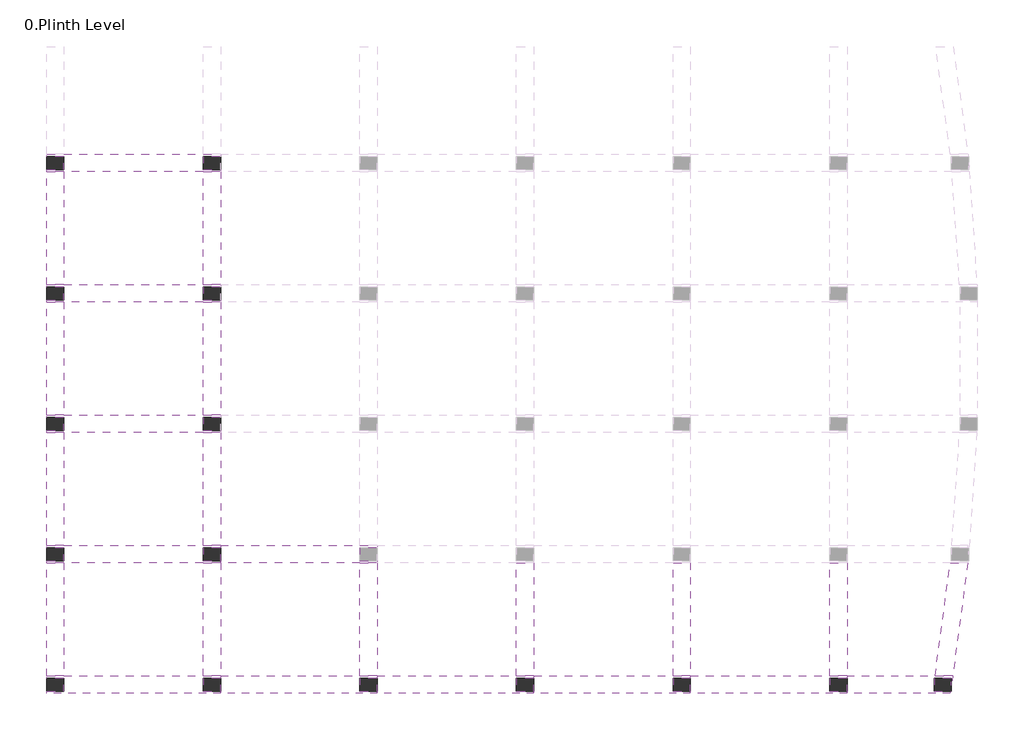
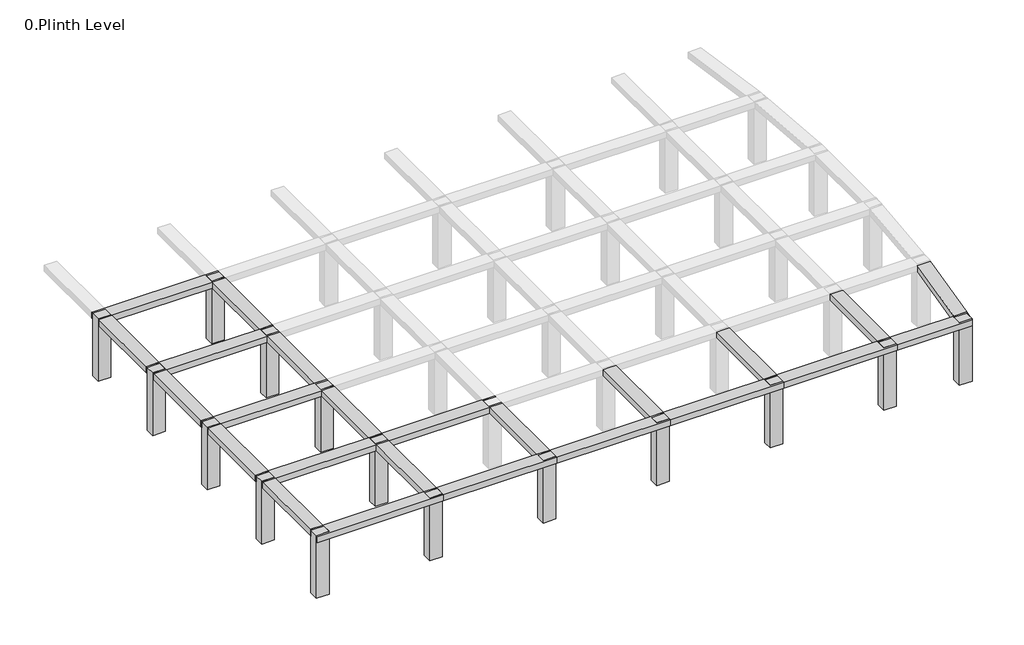
# One storey, part 1 of 3: 24 beams, 15 columns.
"""IFC4 building model written with IfcOpenShell, lengths in millimetres."""

from ifc_helpers import new_model, si_unit, frame, origin, origin_with_axes, place, context, project, spatial, polyline, outline, extrude, faceted_brep, element, save

model = new_model("IFC4")

# Units and contexts
model_context = context("Model", 3, world=origin())
ifc_project = project(units=[si_unit("LENGTHUNIT", "METRE", prefix="MILLI")], contexts=[model_context])

# Site, building, storey
site = spatial("IfcSite", under=ifc_project)
building = spatial("IfcBuilding", under=site)
storey = spatial("IfcBuildingStorey", under=building, Name="0.Plinth Level", Elevation=0.0)

# Beams
placement = place(None, origin())
element("IfcBeam", 1, ObjectType="Concrete-Rectangular Beam : 2' x2'", at=placement, inside=storey, context=model_context, shape_type="Brep", body=[
    faceted_brep([(-16619.274232, -2891.2168778, 3200.4), (-17228.874232, -2891.2168778, 3200.4), (-22105.674232, -2891.2168778, 3200.4), (-22715.274232, -2891.2168778, 3200.4), (-22715.274232, -2967.4168778, 3200.4), (-22105.674232, -2967.4168778, 3200.4), (-22105.674232, -3424.6168778, 3200.4), (-22715.274232, -3424.6168778, 3200.4), (-22715.274232, -3500.8168778, 3200.4), (-16619.274232, -3500.8168778, 3200.4), (-16619.274232, -3424.6168778, 3200.4), (-17228.874232, -3424.6168778, 3200.4), (-17228.874232, -2967.4168778, 3200.4), (-16619.274232, -2967.4168778, 3200.4), (-22715.274232, -3500.8168778, 2895.6), (-16619.274232, -3500.8168778, 2895.6), (-22715.274232, -3424.6168778, 2895.6), (-22105.674232, -3424.6168778, 2895.6), (-22105.674232, -2967.4168778, 2895.6), (-22715.274232, -2967.4168778, 2895.6), (-22715.274232, -2891.2168778, 2895.6), (-22105.674232, -2891.2168778, 2895.6), (-17228.874232, -2891.2168778, 2895.6), (-16619.274232, -2891.2168778, 2895.6), (-16619.274232, -2967.4168778, 2895.6), (-17228.874232, -2967.4168778, 2895.6), (-17228.874232, -3424.6168778, 2895.6), (-16619.274232, -3424.6168778, 2895.6)], [[[0, 1, 2, 3, 4, 5, 6, 7, 8, 9, 10, 11, 12, 13]], [[8, 14, 15, 9]], [[15, 14, 16, 17, 18, 19, 20, 21, 22, 23, 24, 25, 26, 27]], [[20, 3, 2, 1, 0, 23, 22, 21]], [[14, 8, 7, 16]], [[9, 15, 27, 10]], [[17, 6, 5, 18]], [[6, 17, 16, 7]], [[18, 5, 4, 19]], [[3, 20, 19, 4]], [[26, 11, 10, 27]], [[11, 26, 25, 12]], [[12, 25, 24, 13]], [[23, 0, 13, 24]]]),
])
element("IfcBeam", 2, ObjectType="Concrete-Rectangular Beam : 2' x2'", at=placement, inside=storey, context=model_context, shape_type="Brep", body=[
    faceted_brep([(-16619.274232, -2891.2168778, 3200.4), (-16619.274232, -2967.4168778, 3200.4), (-16619.274232, -3424.6168778, 3200.4), (-16619.274232, -3500.8168778, 3200.4), (-11132.874232, -3500.8168778, 3200.4), (-11132.874232, -3424.6168778, 3200.4), (-11742.474232, -3424.6168778, 3200.4), (-11742.474232, -2967.4168778, 3200.4), (-11132.874232, -2967.4168778, 3200.4), (-11132.874232, -2891.2168778, 3200.4), (-11742.474232, -2891.2168778, 3200.4), (-11132.874232, -3500.8168778, 2895.6), (-16619.274232, -3500.8168778, 2895.6), (-16619.274232, -3424.6168778, 2895.6), (-16619.274232, -2967.4168778, 2895.6), (-16619.274232, -2891.2168778, 2895.6), (-11742.474232, -2891.2168778, 2895.6), (-11132.874232, -2891.2168778, 2895.6), (-11132.874232, -2967.4168778, 2895.6), (-11742.474232, -2967.4168778, 2895.6), (-11742.474232, -3424.6168778, 2895.6), (-11132.874232, -3424.6168778, 2895.6)], [[[0, 1, 2, 3, 4, 5, 6, 7, 8, 9, 10]], [[11, 4, 3, 12]], [[12, 13, 14, 15, 16, 17, 18, 19, 20, 21, 11]], [[15, 0, 10, 9, 17, 16]], [[3, 2, 1, 0, 15, 14, 13, 12]], [[4, 11, 21, 5]], [[20, 6, 5, 21]], [[6, 20, 19, 7]], [[7, 19, 18, 8]], [[17, 9, 8, 18]]]),
])
element("IfcBeam", 3, ObjectType="Concrete-Rectangular Beam : 2' x2'", at=placement, inside=storey, context=model_context, shape_type="Brep", body=[
    faceted_brep([(-5646.474232, -2891.2168778, 3200.4), (-6256.074232, -2891.2168778, 3200.4), (-11132.874232, -2891.2168778, 3200.4), (-11132.874232, -2967.4168778, 3200.4), (-11132.874232, -3424.6168778, 3200.4), (-11132.874232, -3500.8168778, 3200.4), (-5646.474232, -3500.8168778, 3200.4), (-5646.474232, -3424.6168778, 3200.4), (-6256.074232, -3424.6168778, 3200.4), (-6256.074232, -2967.4168778, 3200.4), (-5646.474232, -2967.4168778, 3200.4), (-5646.474232, -3500.8168778, 2895.6), (-11132.874232, -3500.8168778, 2895.6), (-11132.874232, -3424.6168778, 2895.6), (-11132.874232, -2967.4168778, 2895.6), (-11132.874232, -2891.2168778, 2895.6), (-6256.074232, -2891.2168778, 2895.6), (-5646.474232, -2891.2168778, 2895.6), (-5646.474232, -2967.4168778, 2895.6), (-6256.074232, -2967.4168778, 2895.6), (-6256.074232, -3424.6168778, 2895.6), (-5646.474232, -3424.6168778, 2895.6)], [[[0, 1, 2, 3, 4, 5, 6, 7, 8, 9, 10]], [[11, 6, 5, 12]], [[11, 12, 13, 14, 15, 16, 17, 18, 19, 20, 21]], [[0, 17, 16, 15, 2, 1]], [[6, 11, 21, 7]], [[5, 4, 3, 2, 15, 14, 13, 12]], [[20, 8, 7, 21]], [[8, 20, 19, 9]], [[9, 19, 18, 10]], [[17, 0, 10, 18]]]),
])
element("IfcBeam", 4, ObjectType="Concrete-Rectangular Beam : 2' x2'", at=placement, inside=storey, context=model_context, shape_type="Brep", body=[
    faceted_brep([(-5646.474232, -2891.2168778, 3200.4), (-5646.474232, -2967.4168778, 3200.4), (-5646.474232, -3424.6168778, 3200.4), (-5646.474232, -3500.8168778, 3200.4), (-160.074232, -3500.8168778, 3200.4), (-160.074232, -3424.6168778, 3200.4), (-769.674232, -3424.6168778, 3200.4), (-769.674232, -2967.4168778, 3200.4), (-160.074232, -2967.4168778, 3200.4), (-160.074232, -2891.2168778, 3200.4), (-769.674232, -2891.2168778, 3200.4), (-160.074232, -3500.8168778, 2895.6), (-5646.474232, -3500.8168778, 2895.6), (-5646.474232, -3424.6168778, 2895.6), (-5646.474232, -2967.4168778, 2895.6), (-5646.474232, -2891.2168778, 2895.6), (-769.674232, -2891.2168778, 2895.6), (-160.074232, -2891.2168778, 2895.6), (-160.074232, -2967.4168778, 2895.6), (-769.674232, -2967.4168778, 2895.6), (-769.674232, -3424.6168778, 2895.6), (-160.074232, -3424.6168778, 2895.6)], [[[0, 1, 2, 3, 4, 5, 6, 7, 8, 9, 10]], [[11, 4, 3, 12]], [[12, 13, 14, 15, 16, 17, 18, 19, 20, 21, 11]], [[15, 0, 10, 9, 17, 16]], [[3, 2, 1, 0, 15, 14, 13, 12]], [[4, 11, 21, 5]], [[20, 6, 5, 21]], [[6, 20, 19, 7]], [[7, 19, 18, 8]], [[17, 9, 8, 18]]]),
])
element("IfcBeam", 5, ObjectType="Concrete-Rectangular Beam : 2' x2'", at=placement, inside=storey, context=model_context, shape_type="Brep", body=[
    faceted_brep([(-160.074232, -2891.2168778, 3200.4), (-160.074232, -2967.4168778, 3200.4), (-160.074232, -3424.6168778, 3200.4), (-160.074232, -3500.8168778, 3200.4), (5326.325768, -3500.8168778, 3200.4), (5326.325768, -3424.6168778, 3200.4), (4716.725768, -3424.6168778, 3200.4), (4716.725768, -2967.4168778, 3200.4), (5326.325768, -2967.4168778, 3200.4), (5326.325768, -2891.2168778, 3200.4), (4716.725768, -2891.2168778, 3200.4), (5326.325768, -3500.8168778, 2895.6), (-160.074232, -3500.8168778, 2895.6), (-160.074232, -3424.6168778, 2895.6), (-160.074232, -2967.4168778, 2895.6), (-160.074232, -2891.2168778, 2895.6), (4716.725768, -2891.2168778, 2895.6), (5326.325768, -2891.2168778, 2895.6), (5326.325768, -2967.4168778, 2895.6), (4716.725768, -2967.4168778, 2895.6), (4716.725768, -3424.6168778, 2895.6), (5326.325768, -3424.6168778, 2895.6)], [[[0, 1, 2, 3, 4, 5, 6, 7, 8, 9, 10]], [[11, 4, 3, 12]], [[12, 13, 14, 15, 16, 17, 18, 19, 20, 21, 11]], [[15, 0, 10, 9, 17, 16]], [[3, 2, 1, 0, 15, 14, 13, 12]], [[4, 11, 21, 5]], [[20, 6, 5, 21]], [[6, 20, 19, 7]], [[7, 19, 18, 8]], [[17, 9, 8, 18]]]),
])
element("IfcBeam", 6, ObjectType="Concrete-Rectangular Beam : 2' x2'", at=placement, inside=storey, context=model_context, shape_type="Brep", body=[
    faceted_brep([(9027.2344863, -2891.2168778, 3200.4), (8412.2463849, -2891.2168778, 3200.4), (5326.325768, -2891.2168778, 3200.4), (5326.325768, -2967.4168778, 3200.4), (5326.325768, -3424.6168778, 3200.4), (5326.325768, -3500.8168778, 3200.4), (8946.005151, -3500.8168778, 3200.4), (8956.158818, -3424.6168778, 3200.4), (8374.325768, -3424.6168778, 3200.4), (8374.325768, -2967.4168778, 3200.4), (8983.925768, -2967.4168778, 3200.4), (8983.925768, -3216.2348608, 3200.4), (8946.005151, -3500.8168778, 2895.6), (5326.325768, -3500.8168778, 2895.6), (5326.325768, -3424.6168778, 2895.6), (5326.325768, -2967.4168778, 2895.6), (5326.325768, -2891.2168778, 2895.6), (8412.2463849, -2891.2168778, 2895.6), (9027.2344863, -2891.2168778, 2895.6), (8983.925768, -3216.2348608, 2895.6), (8983.925768, -2967.4168778, 2895.6), (8374.325768, -2967.4168778, 2895.6), (8374.325768, -3424.6168778, 2895.6), (8956.158818, -3424.6168778, 2895.6)], [[[0, 1, 2, 3, 4, 5, 6, 7, 8, 9, 10, 11]], [[12, 6, 5, 13]], [[12, 13, 14, 15, 16, 17, 18, 19, 20, 21, 22, 23]], [[0, 18, 17, 16, 2, 1]], [[6, 12, 23, 7]], [[5, 4, 3, 2, 16, 15, 14, 13]], [[10, 20, 19, 11]], [[22, 8, 7, 23]], [[8, 22, 21, 9]], [[9, 21, 20, 10]], [[18, 0, 11, 19]]]),
])
element("IfcBeam", 7, ObjectType="Concrete-Rectangular Beam : 2' x2'", at=placement, inside=storey, context=model_context, shape_type="Brep", body=[
    faceted_brep([(-16619.274232, 1680.7831222, 3200.4), (-17228.874232, 1680.7831222, 3200.4), (-22105.674232, 1680.7831222, 3200.4), (-22715.274232, 1680.7831222, 3200.4), (-22715.274232, 1604.5831222, 3200.4), (-22105.674232, 1604.5831222, 3200.4), (-22105.674232, 1147.3831222, 3200.4), (-22715.274232, 1147.3831222, 3200.4), (-22715.274232, 1071.1831222, 3200.4), (-22105.674232, 1071.1831222, 3200.4), (-17228.874232, 1071.1831222, 3200.4), (-16619.274232, 1071.1831222, 3200.4), (-16619.274232, 1147.3831222, 3200.4), (-17228.874232, 1147.3831222, 3200.4), (-17228.874232, 1604.5831222, 3200.4), (-16619.274232, 1604.5831222, 3200.4), (-22715.274232, 1071.1831222, 2895.6), (-22105.674232, 1071.1831222, 2895.6), (-17228.874232, 1071.1831222, 2895.6), (-16619.274232, 1071.1831222, 2895.6), (-22715.274232, 1147.3831222, 2895.6), (-22105.674232, 1147.3831222, 2895.6), (-22105.674232, 1604.5831222, 2895.6), (-22715.274232, 1604.5831222, 2895.6), (-22715.274232, 1680.7831222, 2895.6), (-22105.674232, 1680.7831222, 2895.6), (-17228.874232, 1680.7831222, 2895.6), (-16619.274232, 1680.7831222, 2895.6), (-16619.274232, 1604.5831222, 2895.6), (-17228.874232, 1604.5831222, 2895.6), (-17228.874232, 1147.3831222, 2895.6), (-16619.274232, 1147.3831222, 2895.6)], [[[0, 1, 2, 3, 4, 5, 6, 7, 8, 9, 10, 11, 12, 13, 14, 15]], [[8, 16, 17, 18, 19, 11, 10, 9]], [[19, 18, 17, 16, 20, 21, 22, 23, 24, 25, 26, 27, 28, 29, 30, 31]], [[24, 3, 2, 1, 0, 27, 26, 25]], [[16, 8, 7, 20]], [[11, 19, 31, 12]], [[21, 6, 5, 22]], [[6, 21, 20, 7]], [[22, 5, 4, 23]], [[3, 24, 23, 4]], [[30, 13, 12, 31]], [[13, 30, 29, 14]], [[14, 29, 28, 15]], [[27, 0, 15, 28]]]),
])
element("IfcBeam", 8, ObjectType="Concrete-Rectangular Beam : 2' x2'", at=placement, inside=storey, context=model_context, shape_type="Brep", body=[
    faceted_brep([(-16619.274232, 1680.7831222, 3200.4), (-16619.274232, 1604.5831222, 3200.4), (-16619.274232, 1147.3831222, 3200.4), (-16619.274232, 1071.1831222, 3200.4), (-11742.474232, 1071.1831222, 3200.4), (-11132.874232, 1071.1831222, 3200.4), (-11132.874232, 1147.3831222, 3200.4), (-11742.474232, 1147.3831222, 3200.4), (-11742.474232, 1604.5831222, 3200.4), (-11132.874232, 1604.5831222, 3200.4), (-11132.874232, 1680.7831222, 3200.4), (-11742.474232, 1680.7831222, 3200.4), (-16619.274232, 1071.1831222, 2895.6), (-11742.474232, 1071.1831222, 2895.6), (-11132.874232, 1071.1831222, 2895.6), (-16619.274232, 1147.3831222, 2895.6), (-16619.274232, 1604.5831222, 2895.6), (-16619.274232, 1680.7831222, 2895.6), (-11742.474232, 1680.7831222, 2895.6), (-11132.874232, 1680.7831222, 2895.6), (-11132.874232, 1604.5831222, 2895.6), (-11742.474232, 1604.5831222, 2895.6), (-11742.474232, 1147.3831222, 2895.6), (-11132.874232, 1147.3831222, 2895.6)], [[[0, 1, 2, 3, 4, 5, 6, 7, 8, 9, 10, 11]], [[3, 12, 13, 14, 5, 4]], [[12, 15, 16, 17, 18, 19, 20, 21, 22, 23, 14, 13]], [[10, 19, 18, 17, 0, 11]], [[3, 2, 1, 0, 17, 16, 15, 12]], [[5, 14, 23, 6]], [[22, 7, 6, 23]], [[7, 22, 21, 8]], [[8, 21, 20, 9]], [[19, 10, 9, 20]]]),
])
element("IfcBeam", 9, ObjectType="Concrete-Rectangular Beam : 2' x2'", at=placement, inside=storey, context=model_context, shape_type="Brep", body=[
    faceted_brep([(-16619.274232, 6252.7831222, 3200.4), (-17228.874232, 6252.7831222, 3200.4), (-22105.674232, 6252.7831222, 3200.4), (-22715.274232, 6252.7831222, 3200.4), (-22715.274232, 6176.5831222, 3200.4), (-22105.674232, 6176.5831222, 3200.4), (-22105.674232, 5719.3831222, 3200.4), (-22715.274232, 5719.3831222, 3200.4), (-22715.274232, 5643.1831222, 3200.4), (-22105.674232, 5643.1831222, 3200.4), (-17228.874232, 5643.1831222, 3200.4), (-16619.274232, 5643.1831222, 3200.4), (-16619.274232, 5719.3831222, 3200.4), (-17228.874232, 5719.3831222, 3200.4), (-17228.874232, 6176.5831222, 3200.4), (-16619.274232, 6176.5831222, 3200.4), (-22715.274232, 5643.1831222, 2895.6), (-22105.674232, 5643.1831222, 2895.6), (-17228.874232, 5643.1831222, 2895.6), (-16619.274232, 5643.1831222, 2895.6), (-22715.274232, 5719.3831222, 2895.6), (-22105.674232, 5719.3831222, 2895.6), (-22105.674232, 6176.5831222, 2895.6), (-22715.274232, 6176.5831222, 2895.6), (-22715.274232, 6252.7831222, 2895.6), (-22105.674232, 6252.7831222, 2895.6), (-17228.874232, 6252.7831222, 2895.6), (-16619.274232, 6252.7831222, 2895.6), (-16619.274232, 6176.5831222, 2895.6), (-17228.874232, 6176.5831222, 2895.6), (-17228.874232, 5719.3831222, 2895.6), (-16619.274232, 5719.3831222, 2895.6)], [[[0, 1, 2, 3, 4, 5, 6, 7, 8, 9, 10, 11, 12, 13, 14, 15]], [[8, 16, 17, 18, 19, 11, 10, 9]], [[19, 18, 17, 16, 20, 21, 22, 23, 24, 25, 26, 27, 28, 29, 30, 31]], [[24, 3, 2, 1, 0, 27, 26, 25]], [[16, 8, 7, 20]], [[11, 19, 31, 12]], [[21, 6, 5, 22]], [[6, 21, 20, 7]], [[22, 5, 4, 23]], [[3, 24, 23, 4]], [[30, 13, 12, 31]], [[13, 30, 29, 14]], [[14, 29, 28, 15]], [[27, 0, 15, 28]]]),
])
element("IfcBeam", 10, ObjectType="Concrete-Rectangular Beam : 2' x2'", at=placement, inside=storey, context=model_context, shape_type="Brep", body=[
    faceted_brep([(-16619.274232, 10824.7831222, 3200.4), (-17228.874232, 10824.7831222, 3200.4), (-22105.674232, 10824.7831222, 3200.4), (-22715.274232, 10824.7831222, 3200.4), (-22715.274232, 10748.5831222, 3200.4), (-22105.674232, 10748.5831222, 3200.4), (-22105.674232, 10291.3831222, 3200.4), (-22715.274232, 10291.3831222, 3200.4), (-22715.274232, 10215.1831222, 3200.4), (-22105.674232, 10215.1831222, 3200.4), (-17228.874232, 10215.1831222, 3200.4), (-16619.274232, 10215.1831222, 3200.4), (-16619.274232, 10291.3831222, 3200.4), (-17228.874232, 10291.3831222, 3200.4), (-17228.874232, 10748.5831222, 3200.4), (-16619.274232, 10748.5831222, 3200.4), (-22715.274232, 10215.1831222, 2895.6), (-22105.674232, 10215.1831222, 2895.6), (-17228.874232, 10215.1831222, 2895.6), (-16619.274232, 10215.1831222, 2895.6), (-22715.274232, 10291.3831222, 2895.6), (-22105.674232, 10291.3831222, 2895.6), (-22105.674232, 10748.5831222, 2895.6), (-22715.274232, 10748.5831222, 2895.6), (-22715.274232, 10824.7831222, 2895.6), (-22105.674232, 10824.7831222, 2895.6), (-17228.874232, 10824.7831222, 2895.6), (-16619.274232, 10824.7831222, 2895.6), (-16619.274232, 10748.5831222, 2895.6), (-17228.874232, 10748.5831222, 2895.6), (-17228.874232, 10291.3831222, 2895.6), (-16619.274232, 10291.3831222, 2895.6)], [[[0, 1, 2, 3, 4, 5, 6, 7, 8, 9, 10, 11, 12, 13, 14, 15]], [[8, 16, 17, 18, 19, 11, 10, 9]], [[19, 18, 17, 16, 20, 21, 22, 23, 24, 25, 26, 27, 28, 29, 30, 31]], [[24, 3, 2, 1, 0, 27, 26, 25]], [[16, 8, 7, 20]], [[11, 19, 31, 12]], [[21, 6, 5, 22]], [[6, 21, 20, 7]], [[22, 5, 4, 23]], [[3, 24, 23, 4]], [[30, 13, 12, 31]], [[13, 30, 29, 14]], [[14, 29, 28, 15]], [[27, 0, 15, 28]]]),
])
element("IfcBeam", 11, ObjectType="Concrete-Rectangular Beam : 2' x2'", at=placement, inside=storey, context=model_context, shape_type="Brep", body=[
    faceted_brep([(-16619.274232, 15396.7831222, 3200.4), (-17228.874232, 15396.7831222, 3200.4), (-22105.674232, 15396.7831222, 3200.4), (-22715.274232, 15396.7831222, 3200.4), (-22715.274232, 15320.5831222, 3200.4), (-22105.674232, 15320.5831222, 3200.4), (-22105.674232, 14863.3831222, 3200.4), (-22715.274232, 14863.3831222, 3200.4), (-22715.274232, 14787.1831222, 3200.4), (-22105.674232, 14787.1831222, 3200.4), (-17228.874232, 14787.1831222, 3200.4), (-16619.274232, 14787.1831222, 3200.4), (-16619.274232, 14863.3831222, 3200.4), (-17228.874232, 14863.3831222, 3200.4), (-17228.874232, 15320.5831222, 3200.4), (-16619.274232, 15320.5831222, 3200.4), (-22715.274232, 14787.1831222, 2895.6), (-22105.674232, 14787.1831222, 2895.6), (-17228.874232, 14787.1831222, 2895.6), (-16619.274232, 14787.1831222, 2895.6), (-22715.274232, 14863.3831222, 2895.6), (-22105.674232, 14863.3831222, 2895.6), (-22105.674232, 15320.5831222, 2895.6), (-22715.274232, 15320.5831222, 2895.6), (-22715.274232, 15396.7831222, 2895.6), (-22105.674232, 15396.7831222, 2895.6), (-17228.874232, 15396.7831222, 2895.6), (-16619.274232, 15396.7831222, 2895.6), (-16619.274232, 15320.5831222, 2895.6), (-17228.874232, 15320.5831222, 2895.6), (-17228.874232, 14863.3831222, 2895.6), (-16619.274232, 14863.3831222, 2895.6)], [[[0, 1, 2, 3, 4, 5, 6, 7, 8, 9, 10, 11, 12, 13, 14, 15]], [[8, 16, 17, 18, 19, 11, 10, 9]], [[19, 18, 17, 16, 20, 21, 22, 23, 24, 25, 26, 27, 28, 29, 30, 31]], [[24, 3, 2, 1, 0, 27, 26, 25]], [[16, 8, 7, 20]], [[11, 19, 31, 12]], [[21, 6, 5, 22]], [[6, 21, 20, 7]], [[22, 5, 4, 23]], [[3, 24, 23, 4]], [[30, 13, 12, 31]], [[13, 30, 29, 14]], [[14, 29, 28, 15]], [[27, 0, 15, 28]]]),
])
element("IfcBeam", 12, ObjectType="Concrete-Rectangular Beam : 2' x2'", at=placement, inside=storey, context=model_context, shape_type="SweptSolid", body=[
    extrude(outline(polyline([(-22105.674232, -2891.2168778), (-22715.274232, -2891.2168778), (-22715.274232, 1071.1831222), (-22105.674232, 1071.1831222), (-22105.674232, -2891.2168778)])), frame((0.0, 0.0, 2895.6), z_axis=(0.0, 0.0, 1.0), x_axis=(1.0, 0.0, 0.0)), (0.0, 0.0, 1.0), 304.8),
])
element("IfcBeam", 13, ObjectType="Concrete-Rectangular Beam : 2' x2'", at=placement, inside=storey, context=model_context, shape_type="SweptSolid", body=[
    extrude(outline(polyline([(-22105.674232, 1680.7831222), (-22715.274232, 1680.7831222), (-22715.274232, 5643.1831222), (-22105.674232, 5643.1831222), (-22105.674232, 1680.7831222)])), frame((0.0, 0.0, 2895.6), z_axis=(0.0, 0.0, 1.0), x_axis=(1.0, 0.0, 0.0)), (0.0, 0.0, 1.0), 304.8),
])
element("IfcBeam", 14, ObjectType="Concrete-Rectangular Beam : 2' x2'", at=placement, inside=storey, context=model_context, shape_type="SweptSolid", body=[
    extrude(outline(polyline([(-22105.674232, 6252.7831222), (-22715.274232, 6252.7831222), (-22715.274232, 10215.1831222), (-22105.674232, 10215.1831222), (-22105.674232, 6252.7831222)])), frame((0.0, 0.0, 2895.6), z_axis=(0.0, 0.0, 1.0), x_axis=(1.0, 0.0, 0.0)), (0.0, 0.0, 1.0), 304.8),
])
element("IfcBeam", 15, ObjectType="Concrete-Rectangular Beam : 2' x2'", at=placement, inside=storey, context=model_context, shape_type="SweptSolid", body=[
    extrude(outline(polyline([(-22105.674232, 10824.7831222), (-22715.274232, 10824.7831222), (-22715.274232, 14787.1831222), (-22105.674232, 14787.1831222), (-22105.674232, 10824.7831222)])), frame((0.0, 0.0, 2895.6), z_axis=(0.0, 0.0, 1.0), x_axis=(1.0, 0.0, 0.0)), (0.0, 0.0, 1.0), 304.8),
])
element("IfcBeam", 16, ObjectType="Concrete-Rectangular Beam : 2' x2'", at=placement, inside=storey, context=model_context, shape_type="SweptSolid", body=[
    extrude(outline(polyline([(-17228.874232, 1071.1831222), (-16619.274232, 1071.1831222), (-16619.274232, -2891.2168778), (-17228.874232, -2891.2168778), (-17228.874232, 1071.1831222)])), frame((0.0, 0.0, 2895.6), z_axis=(0.0, 0.0, 1.0), x_axis=(1.0, 0.0, 0.0)), (0.0, 0.0, 1.0), 304.8),
])
element("IfcBeam", 17, ObjectType="Concrete-Rectangular Beam : 2' x2'", at=placement, inside=storey, context=model_context, shape_type="SweptSolid", body=[
    extrude(outline(polyline([(-16619.274232, 1680.7831222), (-17228.874232, 1680.7831222), (-17228.874232, 5643.1831222), (-16619.274232, 5643.1831222), (-16619.274232, 1680.7831222)])), frame((0.0, 0.0, 2895.6), z_axis=(0.0, 0.0, 1.0), x_axis=(1.0, 0.0, 0.0)), (0.0, 0.0, 1.0), 304.8),
])
element("IfcBeam", 18, ObjectType="Concrete-Rectangular Beam : 2' x2'", at=placement, inside=storey, context=model_context, shape_type="SweptSolid", body=[
    extrude(outline(polyline([(-16619.274232, 6252.7831222), (-17228.874232, 6252.7831222), (-17228.874232, 10215.1831222), (-16619.274232, 10215.1831222), (-16619.274232, 6252.7831222)])), frame((0.0, 0.0, 2895.6), z_axis=(0.0, 0.0, 1.0), x_axis=(1.0, 0.0, 0.0)), (0.0, 0.0, 1.0), 304.8),
])
element("IfcBeam", 19, ObjectType="Concrete-Rectangular Beam : 2' x2'", at=placement, inside=storey, context=model_context, shape_type="SweptSolid", body=[
    extrude(outline(polyline([(-16619.274232, 10824.7831222), (-17228.874232, 10824.7831222), (-17228.874232, 14787.1831222), (-16619.274232, 14787.1831222), (-16619.274232, 10824.7831222)])), frame((0.0, 0.0, 2895.6), z_axis=(0.0, 0.0, 1.0), x_axis=(1.0, 0.0, 0.0)), (0.0, 0.0, 1.0), 304.8),
])
element("IfcBeam", 20, ObjectType="Concrete-Rectangular Beam : 2' x2'", at=placement, inside=storey, context=model_context, shape_type="SweptSolid", body=[
    extrude(outline(polyline([(-11742.474232, 1071.1831222), (-11132.874232, 1071.1831222), (-11132.874232, -2891.2168778), (-11742.474232, -2891.2168778), (-11742.474232, 1071.1831222)])), frame((0.0, 0.0, 2895.6), z_axis=(0.0, 0.0, 1.0), x_axis=(1.0, 0.0, 0.0)), (0.0, 0.0, 1.0), 304.8),
])
element("IfcBeam", 21, ObjectType="Concrete-Rectangular Beam : 2' x2'", at=placement, inside=storey, context=model_context, shape_type="SweptSolid", body=[
    extrude(outline(polyline([(-6256.074232, 1071.1831222), (-5646.474232, 1071.1831222), (-5646.474232, -2891.2168778), (-6256.074232, -2891.2168778), (-6256.074232, 1071.1831222)])), frame((0.0, 0.0, 2895.6), z_axis=(0.0, 0.0, 1.0), x_axis=(1.0, 0.0, 0.0)), (0.0, 0.0, 1.0), 304.8),
])
element("IfcBeam", 22, ObjectType="Concrete-Rectangular Beam : 2' x2'", at=placement, inside=storey, context=model_context, shape_type="SweptSolid", body=[
    extrude(outline(polyline([(-769.674232, 1071.1831222), (-160.074232, 1071.1831222), (-160.074232, -2891.2168778), (-769.674232, -2891.2168778), (-769.674232, 1071.1831222)])), frame((0.0, 0.0, 2895.6), z_axis=(0.0, 0.0, 1.0), x_axis=(1.0, 0.0, 0.0)), (0.0, 0.0, 1.0), 304.8),
])
element("IfcBeam", 23, ObjectType="Concrete-Rectangular Beam : 2' x2'", at=placement, inside=storey, context=model_context, shape_type="SweptSolid", body=[
    extrude(outline(polyline([(4716.725768, 1071.1831222), (5326.325768, 1071.1831222), (5326.325768, -2891.2168778), (4716.725768, -2891.2168778), (4716.725768, 1071.1831222)])), frame((0.0, 0.0, 2895.6), z_axis=(0.0, 0.0, 1.0), x_axis=(1.0, 0.0, 0.0)), (0.0, 0.0, 1.0), 304.8),
])
element("IfcBeam", 24, ObjectType="Concrete-Rectangular Beam : 2' x2'", at=placement, inside=storey, context=model_context, shape_type="SweptSolid", body=[
    extrude(outline(polyline([(8940.2370643, 1071.1831222), (9555.2251658, 1071.1831222), (9027.2344863, -2891.2168778), (8412.2463849, -2891.2168778), (8940.2370643, 1071.1831222)])), frame((0.0, 0.0, 2895.6), z_axis=(0.0, 0.0, 1.0), x_axis=(1.0, 0.0, 0.0)), (0.0, 0.0, 1.0), 304.8),
])

# Columns
element("IfcColumn", 25, ObjectType="Concrete-Rectangular-Column : 12 x 18", at=placement, inside=storey, context=model_context, shape_type="SweptSolid", body=[
    extrude(outline(polyline([(-22105.674232, -2967.4168778), (-22105.674232, -3424.6168778), (-22715.274232, -3424.6168778), (-22715.274232, -2967.4168778), (-22105.674232, -2967.4168778)])), origin_with_axes(), (0.0, 0.0, 1.0), 3200.4),
])
element("IfcColumn", 26, ObjectType="Concrete-Rectangular-Column : 12 x 18", at=placement, inside=storey, context=model_context, shape_type="SweptSolid", body=[
    extrude(outline(polyline([(-16619.274232, -2967.4168778), (-16619.274232, -3424.6168778), (-17228.874232, -3424.6168778), (-17228.874232, -2967.4168778), (-16619.274232, -2967.4168778)])), origin_with_axes(), (0.0, 0.0, 1.0), 3200.4),
])
element("IfcColumn", 27, ObjectType="Concrete-Rectangular-Column : 12 x 18", at=placement, inside=storey, context=model_context, shape_type="SweptSolid", body=[
    extrude(outline(polyline([(-11132.874232, -2967.4168778), (-11132.874232, -3424.6168778), (-11742.474232, -3424.6168778), (-11742.474232, -2967.4168778), (-11132.874232, -2967.4168778)])), origin_with_axes(), (0.0, 0.0, 1.0), 3200.4),
])
element("IfcColumn", 28, ObjectType="Concrete-Rectangular-Column : 12 x 18", at=placement, inside=storey, context=model_context, shape_type="SweptSolid", body=[
    extrude(outline(polyline([(-5646.474232, -2967.4168778), (-5646.474232, -3424.6168778), (-6256.074232, -3424.6168778), (-6256.074232, -2967.4168778), (-5646.474232, -2967.4168778)])), origin_with_axes(), (0.0, 0.0, 1.0), 3200.4),
])
element("IfcColumn", 29, ObjectType="Concrete-Rectangular-Column : 12 x 18", at=placement, inside=storey, context=model_context, shape_type="SweptSolid", body=[
    extrude(outline(polyline([(-160.074232, -2967.4168778), (-160.074232, -3424.6168778), (-769.674232, -3424.6168778), (-769.674232, -2967.4168778), (-160.074232, -2967.4168778)])), origin_with_axes(), (0.0, 0.0, 1.0), 3200.4),
])
element("IfcColumn", 30, ObjectType="Concrete-Rectangular-Column : 12 x 18", at=placement, inside=storey, context=model_context, shape_type="SweptSolid", body=[
    extrude(outline(polyline([(5326.325768, -2967.4168778), (5326.325768, -3424.6168778), (4716.725768, -3424.6168778), (4716.725768, -2967.4168778), (5326.325768, -2967.4168778)])), origin_with_axes(), (0.0, 0.0, 1.0), 3200.4),
])
element("IfcColumn", 31, ObjectType="Concrete-Rectangular-Column : 12 x 18", at=placement, inside=storey, context=model_context, shape_type="SweptSolid", body=[
    extrude(outline(polyline([(8983.925768, -2967.4168778), (8983.925768, -3424.6168778), (8374.325768, -3424.6168778), (8374.325768, -2967.4168778), (8983.925768, -2967.4168778)])), origin_with_axes(), (0.0, 0.0, 1.0), 3200.4),
])
element("IfcColumn", 32, ObjectType="Concrete-Rectangular-Column : 12 x 18", at=placement, inside=storey, context=model_context, shape_type="SweptSolid", body=[
    extrude(outline(polyline([(-22105.674232, 1604.5831222), (-22105.674232, 1147.3831222), (-22715.274232, 1147.3831222), (-22715.274232, 1604.5831222), (-22105.674232, 1604.5831222)])), origin_with_axes(), (0.0, 0.0, 1.0), 3200.4),
])
element("IfcColumn", 33, ObjectType="Concrete-Rectangular-Column : 12 x 18", at=placement, inside=storey, context=model_context, shape_type="SweptSolid", body=[
    extrude(outline(polyline([(-16619.274232, 1604.5831222), (-16619.274232, 1147.3831222), (-17228.874232, 1147.3831222), (-17228.874232, 1604.5831222), (-16619.274232, 1604.5831222)])), origin_with_axes(), (0.0, 0.0, 1.0), 3200.4),
])
element("IfcColumn", 34, ObjectType="Concrete-Rectangular-Column : 12 x 18", at=placement, inside=storey, context=model_context, shape_type="SweptSolid", body=[
    extrude(outline(polyline([(-22105.674232, 6176.5831222), (-22105.674232, 5719.3831222), (-22715.274232, 5719.3831222), (-22715.274232, 6176.5831222), (-22105.674232, 6176.5831222)])), origin_with_axes(), (0.0, 0.0, 1.0), 3200.4),
])
element("IfcColumn", 35, ObjectType="Concrete-Rectangular-Column : 12 x 18", at=placement, inside=storey, context=model_context, shape_type="SweptSolid", body=[
    extrude(outline(polyline([(-16619.274232, 6176.5831222), (-16619.274232, 5719.3831222), (-17228.874232, 5719.3831222), (-17228.874232, 6176.5831222), (-16619.274232, 6176.5831222)])), origin_with_axes(), (0.0, 0.0, 1.0), 3200.4),
])
element("IfcColumn", 36, ObjectType="Concrete-Rectangular-Column : 12 x 18", at=placement, inside=storey, context=model_context, shape_type="SweptSolid", body=[
    extrude(outline(polyline([(-22105.674232, 10748.5831222), (-22105.674232, 10291.3831222), (-22715.274232, 10291.3831222), (-22715.274232, 10748.5831222), (-22105.674232, 10748.5831222)])), origin_with_axes(), (0.0, 0.0, 1.0), 3200.4),
])
element("IfcColumn", 37, ObjectType="Concrete-Rectangular-Column : 12 x 18", at=placement, inside=storey, context=model_context, shape_type="SweptSolid", body=[
    extrude(outline(polyline([(-16619.274232, 10748.5831222), (-16619.274232, 10291.3831222), (-17228.874232, 10291.3831222), (-17228.874232, 10748.5831222), (-16619.274232, 10748.5831222)])), origin_with_axes(), (0.0, 0.0, 1.0), 3200.4),
])
element("IfcColumn", 38, ObjectType="Concrete-Rectangular-Column : 12 x 18", at=placement, inside=storey, context=model_context, shape_type="SweptSolid", body=[
    extrude(outline(polyline([(-22105.674232, 15320.5831222), (-22105.674232, 14863.3831222), (-22715.274232, 14863.3831222), (-22715.274232, 15320.5831222), (-22105.674232, 15320.5831222)])), origin_with_axes(), (0.0, 0.0, 1.0), 3200.4),
])
element("IfcColumn", 39, ObjectType="Concrete-Rectangular-Column : 12 x 18", at=placement, inside=storey, context=model_context, shape_type="SweptSolid", body=[
    extrude(outline(polyline([(-16619.274232, 15320.5831222), (-16619.274232, 14863.3831222), (-17228.874232, 14863.3831222), (-17228.874232, 15320.5831222), (-16619.274232, 15320.5831222)])), origin_with_axes(), (0.0, 0.0, 1.0), 3200.4),
])

save(model, "model.ifc")

# Revit data of these elements
# Type "Concrete-Rectangular Beam : 2' x2'"
#   Assembly Code = "B10"
#   Length [instance default] = 5' - 0"
#   b = 2' - 0"
#   h = 1' - 0"
#   Structural Material [instance default] = Concrete, Cast-in-Place gray
# Type "Concrete-Rectangular-Column : 12 x 18"
#   Assembly Code = "B10"
#   b = 2' - 0"
#   h = 1' - 6"
#   Structural Material [instance default] = Concrete, Cast-in-Place gray
# Elements 1, 2, 3, 4, 5, 6, 7, 8, 9, 10, 11, 12, 13, 14, 15, 16, 17, 18, 19, 20, 21, 22, 23, 24 (IfcBeam, "Concrete-Rectangular Beam : 2' x2'")
#   Structural Material = Concrete, Precast (2)
#   Phase Created = New Construction
#   Materials on its faces: "Concrete, Precast (2)"
# Elements 25, 26, 27, 28, 29, 30, 31, 32, 33, 34, 35, 36, 37, 38, 39 (IfcColumn, "Concrete-Rectangular-Column : 12 x 18")
#   Phase Created = New Construction
#   Materials on its faces: "Concrete, Cast-in-Place gray"
# Materials
#   "Concrete, Cast-in-Place gray": class "Concrete", colour RGB 192 192 192, transparency 0, Description = "Cast-in-place concrete", Cost = 0
#   "Concrete, Precast (2)": class "Concrete", colour RGB 198 187 187, transparency 0, Description = "Precast concrete", Cost = 0
